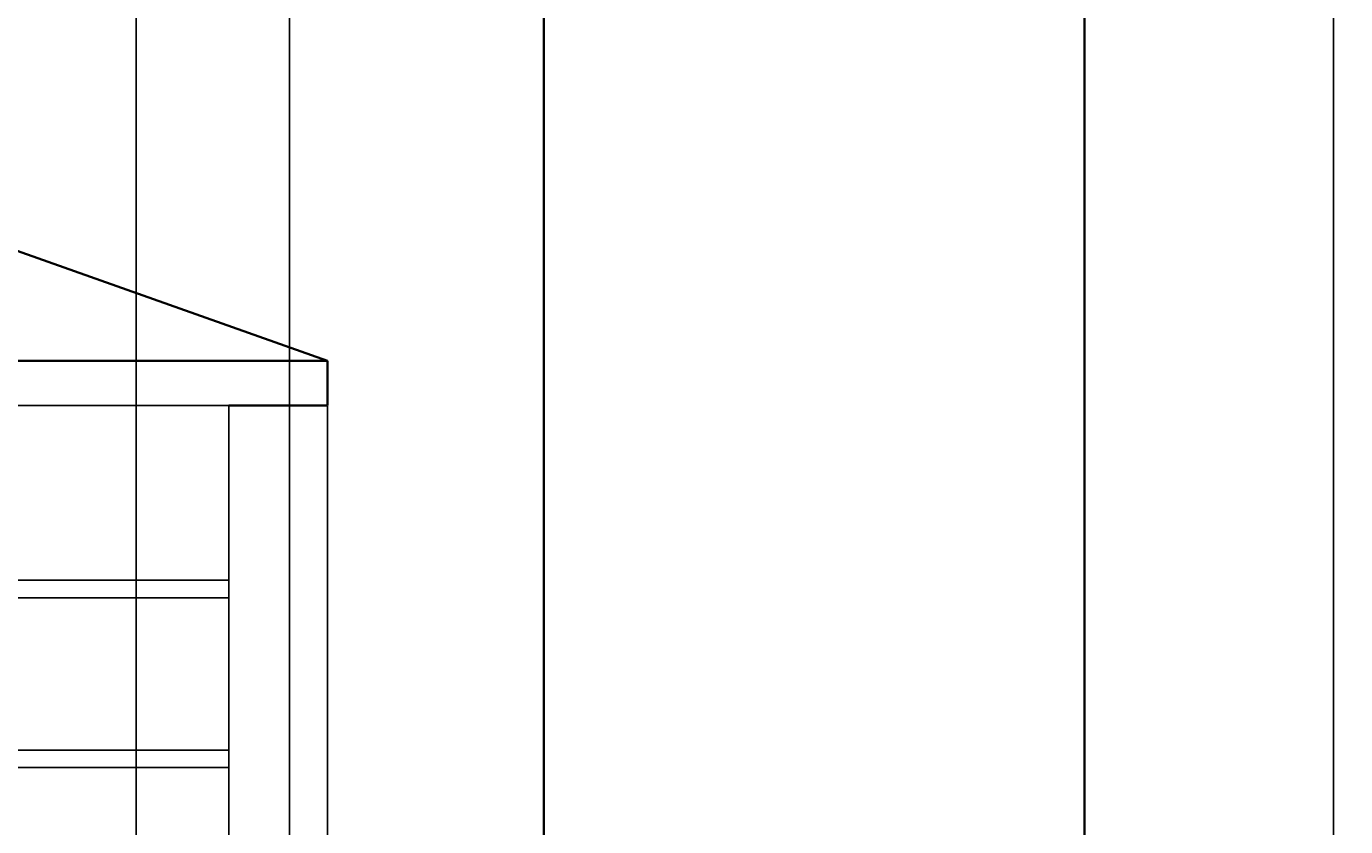
# Model space of a CAD drawing. Units: inches. Extents: x 69 to 650, y -16 to 573.
# Tile 10 of 26: x 499 to 649, y 126 to 218. Entities that reach past the tile are written whole.
import ezdxf

# ---------------------------------------------------------------- set-up
doc = ezdxf.new("R2010")
doc.units = ezdxf.units.IN
doc.header["$MEASUREMENT"] = 0
for name, color, linetype, lineweight in [('A-ANNO-DIMS', 2, 'Continuous', 18), ('A-COLS', 7, 'Continuous', 25), ('A-ROOF', 7, 'Continuous', 35), ('A-WALL', 7, 'Continuous', 35)]:
    doc.layers.add(name, color=color, linetype=linetype, lineweight=lineweight)
doc.styles.get("Standard").update_dxf_attribs({"font": 'arial.ttf'})
doc.dimstyles.get("Standard").update_dxf_attribs({"dimtxt": 0.8125, "dimasz": 0.18, "dimexe": 0.18, "dimexo": 0.0625, "dimgap": 0.09, "dimtad": 0, "dimtih": 1, "dimtoh": 1, "dimdec": 4, "dimzin": 0, "dimdsep": 46, "dimlunit": 4, "dimtxsty": 'Standard', "dimcen": 0.09, "dimadec": 0, "dimazin": 0, "dimtfac": 1, "dimtdec": 4, "dimtofl": 0, "dimtmove": 0, "dimatfit": 3, "dimfxl": 1, "dimtolj": 1, "dimtzin": 0, "dimarcsym": 0})

# ---------------------------------------------------------------- blocks, each defined once
blk = doc.blocks.new('PIER-PORTAL-BANDED')
for p, q in [((0, 0), (0, 86.34)), ((0, 86.34), (26.94, 86.34)), ((0, 66.41), (26.94, 66.41)), ((0, 64.41), (26.94, 64.41)), ((0, 47.05), (26.94, 47.05)), ((0, 45.05), (26.94, 45.05)), ((0, 28.76), (26.94, 28.76)), ((0, 26.76), (26.94, 26.76)), ((0, 11.45), (26.94, 11.45)), ((0, 9.45), (26.94, 9.45))]:
    blk.add_line(p, q)
blk = doc.blocks.new('*D19')
at = {"layer": 'A-ANNO-DIMS', "color": 0, "lineweight": -2, "transparency": 16777216}
for p, q in [((99.56, 471.72), (99.56, 572.74)), ((99.74, 572.56), (358.57, 572.56)), ((619.38, 572.56), (360.54, 572.56)), ((619.56, 87.99), (619.56, 572.74))]:
    blk.add_line(p, q, dxfattribs=at)
at = {"layer": 'A-ANNO-DIMS', "color": 0, "transparency": 16777216}
for points in [[(99.74, 572.59), (99.74, 572.53), (99.56, 572.56)], [(619.38, 572.59), (619.38, 572.53), (619.56, 572.56)]]:
    blk.add_solid(points, dxfattribs=at)
at = {"layer": 'Defpoints', "color": 0, "transparency": 16777216}
for p in [(619.56, 572.56), (99.56, 471.66), (619.56, 87.93)]:
    blk.add_point(p, dxfattribs=at)
at = {"layer": 'A-ANNO-DIMS', "color": 0, "transparency": 16777216, "insert": (359.56, 572.56), "char_height": 0.812, "attachment_point": 5}
blk.add_mtext('\\A1;520', dxfattribs=at)
blk = doc.blocks.new('*D20')
at = {"layer": 'A-ANNO-DIMS', "color": 0, "lineweight": -2, "transparency": 16777216}
for p, q in [((504.24, 544.16), (648.14, 544.16)), ((647.96, 543.98), (647.96, 304.55)), ((647.96, 64.11), (647.96, 303.54)), ((619.62, 63.93), (648.14, 63.93))]:
    blk.add_line(p, q, dxfattribs=at)
at = {"layer": 'A-ANNO-DIMS', "color": 0, "transparency": 16777216}
for points in [[(647.93, 543.98), (647.99, 543.98), (647.96, 544.16)], [(647.93, 64.11), (647.99, 64.11), (647.96, 63.93)]]:
    blk.add_solid(points, dxfattribs=at)
at = {"layer": 'Defpoints', "color": 0, "transparency": 16777216}
for p in [(504.18, 544.16), (647.96, 544.16), (619.56, 63.93)]:
    blk.add_point(p, dxfattribs=at)
at = {"layer": 'A-ANNO-DIMS', "color": 0, "transparency": 16777216, "insert": (647.96, 304.04), "char_height": 0.812, "attachment_point": 5}
blk.add_mtext('\\A1;480.2', dxfattribs=at)
blk = doc.blocks.new('*D33')
at = {"layer": 'A-ANNO-DIMS', "color": 0, "lineweight": -2, "transparency": 16777216}
for p, q in [((533.14, 174.2), (533.14, 35.35)), ((521.86, 87.87), (521.86, 35.35)), ((522.04, 35.53), (526.07, 35.53)), ((532.96, 35.53), (528.92, 35.53))]:
    blk.add_line(p, q, dxfattribs=at)
at = {"layer": 'A-ANNO-DIMS', "color": 0, "transparency": 16777216}
for points in [[(522.04, 35.56), (522.04, 35.5), (521.86, 35.53)], [(532.96, 35.56), (532.96, 35.5), (533.14, 35.53)]]:
    blk.add_solid(points, dxfattribs=at)
at = {"layer": 'Defpoints', "color": 0, "transparency": 16777216}
for p in [(533.14, 174.27), (521.86, 87.93), (533.14, 35.53)]:
    blk.add_point(p, dxfattribs=at)
at = {"layer": 'A-ANNO-DIMS', "color": 0, "transparency": 16777216, "insert": (527.5, 35.53), "char_height": 0.812, "attachment_point": 5}
blk.add_mtext('\\A1;11.28', dxfattribs=at)
blk = doc.blocks.new('*D34')
at = {"layer": 'A-ANNO-DIMS', "color": 0, "lineweight": -2, "transparency": 16777216}
for p, q in [((533.14, 174.2), (533.14, 35.35)), ((619.56, 87.87), (619.56, 35.35)), ((533.32, 35.53), (574.89, 35.53)), ((619.38, 35.53), (577.8, 35.53))]:
    blk.add_line(p, q, dxfattribs=at)
at = {"layer": 'A-ANNO-DIMS', "color": 0, "transparency": 16777216}
for points in [[(533.32, 35.56), (533.32, 35.5), (533.14, 35.53)], [(619.38, 35.56), (619.38, 35.5), (619.56, 35.53)]]:
    blk.add_solid(points, dxfattribs=at)
at = {"layer": 'Defpoints', "color": 0, "transparency": 16777216}
for p in [(533.14, 174.27), (619.56, 87.93), (619.56, 35.53)]:
    blk.add_point(p, dxfattribs=at)
at = {"layer": 'A-ANNO-DIMS', "color": 0, "transparency": 16777216, "insert": (576.35, 35.53), "char_height": 0.812, "attachment_point": 5}
blk.add_mtext('\\A1;86.42', dxfattribs=at)
blk = doc.blocks.new('*D40')
at = {"layer": 'A-ANNO-DIMS', "color": 0, "lineweight": -2, "transparency": 16777216}
for p, q in [((511.3, 372.93), (511.3, 35.35)), ((528.81, 243.87), (528.81, 35.35)), ((511.48, 35.53), (518.32, 35.53)), ((528.63, 35.53), (521.79, 35.53))]:
    blk.add_line(p, q, dxfattribs=at)
at = {"layer": 'A-ANNO-DIMS', "color": 0, "transparency": 16777216}
for points in [[(511.48, 35.56), (511.48, 35.5), (511.3, 35.53)], [(528.63, 35.56), (528.63, 35.5), (528.81, 35.53)]]:
    blk.add_solid(points, dxfattribs=at)
at = {"layer": 'Defpoints', "color": 0, "transparency": 16777216}
for p in [(511.3, 372.99), (528.81, 243.93), (528.81, 35.53)]:
    blk.add_point(p, dxfattribs=at)
at = {"layer": 'A-ANNO-DIMS', "color": 0, "transparency": 16777216, "insert": (520.06, 35.53), "char_height": 0.812, "attachment_point": 5}
blk.add_mtext('\\A1;17.514', dxfattribs=at)
blk = doc.blocks.new('*D41')
at = {"layer": 'A-ANNO-DIMS', "color": 0, "lineweight": -2, "transparency": 16777216}
for p, q in [((528.81, 243.87), (528.81, 35.35)), ((619.56, 243.87), (619.56, 35.35)), ((528.99, 35.53), (572.72, 35.53)), ((619.38, 35.53), (575.64, 35.53))]:
    blk.add_line(p, q, dxfattribs=at)
at = {"layer": 'A-ANNO-DIMS', "color": 0, "transparency": 16777216}
for points in [[(528.99, 35.56), (528.99, 35.5), (528.81, 35.53)], [(619.38, 35.56), (619.38, 35.5), (619.56, 35.53)]]:
    blk.add_solid(points, dxfattribs=at)
at = {"layer": 'Defpoints', "color": 0, "transparency": 16777216}
for p in [(528.81, 243.93), (619.56, 243.93), (619.56, 35.53)]:
    blk.add_point(p, dxfattribs=at)
at = {"layer": 'A-ANNO-DIMS', "color": 0, "transparency": 16777216, "insert": (574.18, 35.53), "char_height": 0.812, "attachment_point": 5}
blk.add_mtext('\\A1;90.74', dxfattribs=at)

msp = doc.modelspace()

# ---------------------------------------------------------------- linework, layer by layer
at = {"layer": 'A-ROOF'}
for p, q in [((441.9398, 211.6519), (533.1369, 179.3737)), ((352.9415, 179.3737), (533.1369, 179.3737)), ((533.1369, 179.3737), (533.1369, 174.2666)), ((533.1369, 174.2666), (521.8566, 174.2666))]:
    msp.add_line(p, q, dxfattribs=at)
at = {"layer": 'A-WALL'}
for p, q in [((619.555, 411.93), (619.555, 69.3788)), ((557.8179, 243.93), (557.8179, 87.93))]:
    msp.add_line(p, q, dxfattribs=at)

# ---------------------------------------------------------------- block references
at = {"layer": 'A-COLS', "extrusion": (0, 0, -1), "zscale": -1}
msp.add_blockref('PIER-PORTAL-BANDED', (-521.8566, 87.93), dxfattribs=at)

# ---------------------------------------------------------------- dimensions: what is measured, and where the dimension line sits
at = {"layer": 'A-ANNO-DIMS'}
for base, p1, p2, override, picture, middle in [((619.555, 572.5573), (99.556, 471.6595), (619.555, 87.93), {"dimdec": 0, "dimlfac": 1, "dimrnd": 0, "dimzin": 0, "dimdsep": 46, "dimlunit": 2}, '*D19', (359.5555, 572.5573)), ((528.812, 35.53), (511.2984, 372.9907), (528.812, 243.93), {"dimdec": 3, "dimlfac": 1, "dimrnd": 0, "dimzin": 0, "dimdsep": 46, "dimlunit": 2}, '*D40', (520.0552, 35.53)), ((619.555, 35.53), (528.812, 243.93), (619.555, 243.93), {"dimdec": 2, "dimlfac": 1, "dimrnd": 0, "dimzin": 0, "dimdsep": 46, "dimlunit": 2}, '*D41', (574.1835, 35.53)), ((533.1369, 35.53), (521.8566, 87.93), (533.1369, 174.2666), {"dimdec": 2, "dimlfac": 1, "dimrnd": 0, "dimzin": 0, "dimdsep": 46, "dimlunit": 2}, '*D33', (527.4967, 35.53)), ((619.555, 35.53), (533.1369, 174.2666), (619.555, 87.93), {"dimdec": 2, "dimlfac": 1, "dimrnd": 0, "dimzin": 0, "dimdsep": 46, "dimlunit": 2}, '*D34', (576.3459, 35.53))]:
    dim = msp.add_linear_dim(base=base, p1=p1, p2=p2, dimstyle='Standard', override=override, dxfattribs=at)
    dim.commit()
    dim.dimension.update_dxf_attribs({"geometry": picture, "text_midpoint": middle})
dim = msp.add_linear_dim(base=(647.955, 544.1573), p1=(619.555, 63.93), p2=(504.1763, 544.1573), angle=90, dimstyle='Standard', override={"dimdec": 1, "dimlfac": 1, "dimrnd": 0, "dimzin": 0, "dimdsep": 46, "dimlunit": 2}, dxfattribs=at)
dim.commit()
dim.dimension.update_dxf_attribs({"geometry": '*D20', "text_midpoint": (647.955, 304.0436)})

doc.saveas('drawing.dxf')
